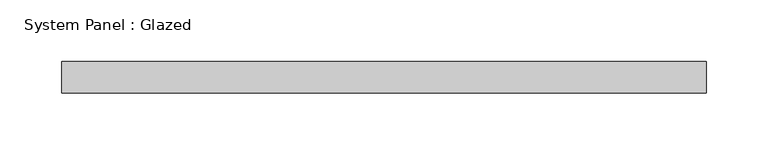
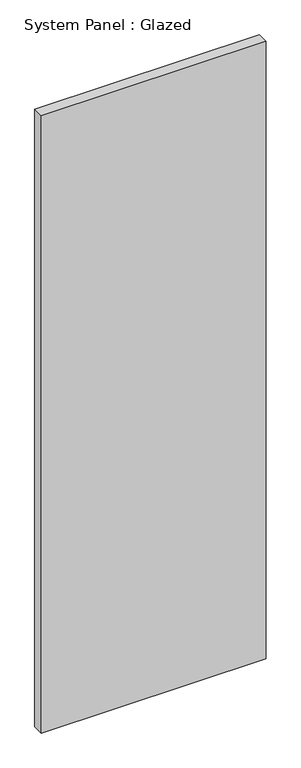
"""IFC4 building model written with IfcOpenShell, lengths in millimetres: plate geometry, System Panel : Glazed."""

from ifc_helpers import new_model, si_unit, origin, origin_with_axes, place, context, project, spatial, polyline, outline, extrude, source, transform, mapped, element, save


def system_panel_glazed_bf89bbd2(model_context):
    return source(origin(), model_context, "Body", "SweptSolid", [
        extrude(outline(polyline([(260.35, 19.05), (-260.35, 19.05), (-260.35, 44.45), (260.35, 44.45), (260.35, 19.05)])), origin_with_axes(), (0.0, 0.0, 1.0), 1509.844519),
    ])


if __name__ == "__main__":
    model = new_model("IFC4")
    model_context = context("Model", 3, world=origin())
    ifc_project = project(units=[si_unit("LENGTHUNIT", "METRE", prefix="MILLI")], contexts=[model_context])
    site = spatial("IfcSite", under=ifc_project)
    building = spatial("IfcBuilding", under=site)
    placement = place(None, origin())
    system_panel_glazed_shape = system_panel_glazed_bf89bbd2(model_context)
    element("IfcPlate", 1, ObjectType="System Panel : Glazed", at=placement, inside=building, context=model_context, shape_type="MappedRepresentation", body=[
        mapped(system_panel_glazed_shape, transform((0.0, 0.0, 0.0), x_axis=(1.0, 0.0, 0.0), y_axis=(0.0, 1.0, 0.0), z_axis=(0.0, 0.0, 1.0))),
    ])
    save(model, "model.ifc")

# Revit data of these elements
# Type "System Panel : Glazed"
#   Construction Type Id = "GSP4R"
#   Analytic Construction = "1/8 in Pilkington single glazing"
#   Visual Light Transmittance = 0.9
#   Solar Heat Gain Coefficient = 0.86
#   Heat Transfer Coefficient (U) = 1.18115 BTU/(h·ft²·°F)
#   Define Thermal Properties by = 1
# Element 1 (IfcPlate, "System Panel : Glazed")
#   Materials on its faces: "Glass"
# Materials
#   "Glass": class "Glass", colour RGB 0 128 192, transparency 0.75, Description = "Soda Lime Glass", Cost = 0
